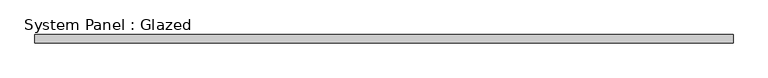
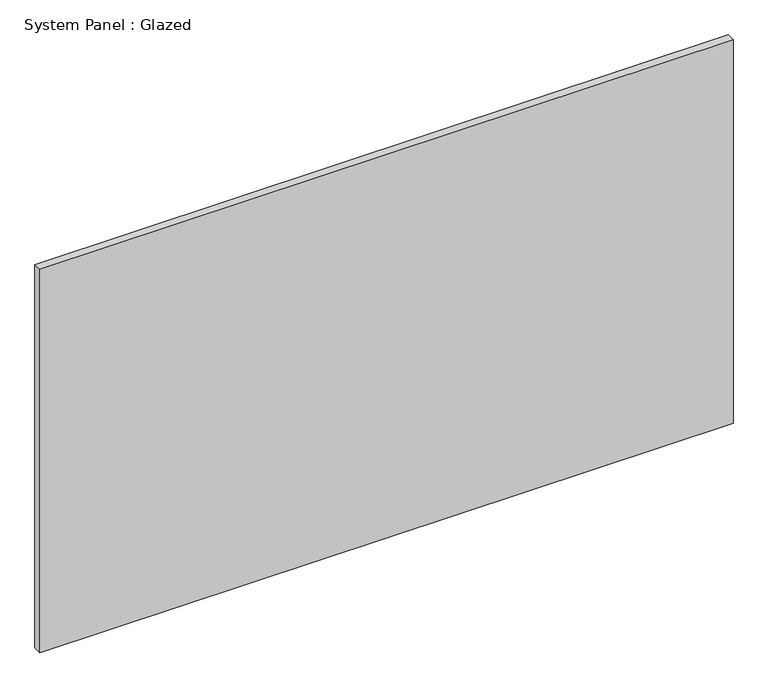
"""IFC4 building model written with IfcOpenShell, lengths in millimetres: plate geometry, System Panel : Glazed."""

from ifc_helpers import new_model, si_unit, origin, origin_with_axes, place, context, project, spatial, polyline, outline, extrude, source, transform, mapped, element, save


def system_panel_glazed_6865593f(model_context):
    return source(origin(), model_context, "Body", "SweptSolid", [
        extrude(outline(polyline([(1042.682696, 19.05), (-1042.682696, 19.05), (-1042.682696, 44.45), (1042.682696, 44.45), (1042.682696, 19.05)])), origin_with_axes(), (0.0, 0.0, 1.0), 1219.2),
    ])


if __name__ == "__main__":
    model = new_model("IFC4")
    model_context = context("Model", 3, world=origin())
    ifc_project = project(units=[si_unit("LENGTHUNIT", "METRE", prefix="MILLI")], contexts=[model_context])
    site = spatial("IfcSite", under=ifc_project)
    building = spatial("IfcBuilding", under=site)
    placement = place(None, origin())
    system_panel_glazed_shape = system_panel_glazed_6865593f(model_context)
    element("IfcPlate", 1, ObjectType="System Panel : Glazed", at=placement, inside=building, context=model_context, shape_type="MappedRepresentation", body=[
        mapped(system_panel_glazed_shape, transform((0.0, 0.0, 0.0), x_axis=(1.0, 0.0, 0.0), y_axis=(0.0, 1.0, 0.0), z_axis=(0.0, 0.0, 1.0))),
    ])
    save(model, "model.ifc")

# Revit data of these elements
# Type "System Panel : Glazed"
#   Construction Type Id = "GSP4R"
#   Analytic Construction = "1/8 in Pilkington single glazing"
#   Visual Light Transmittance = 0.9
#   Solar Heat Gain Coefficient = 0.86
#   Heat Transfer Coefficient (U) = 1.18115 BTU/(h·ft²·°F)
# Element 1 (IfcPlate, "System Panel : Glazed")
#   Materials on its faces: "Glass"
# Materials
#   "Glass": class "Glass", colour RGB 0 128 192, transparency 0.75, Description = "Soda Lime Glass", Cost = 0
